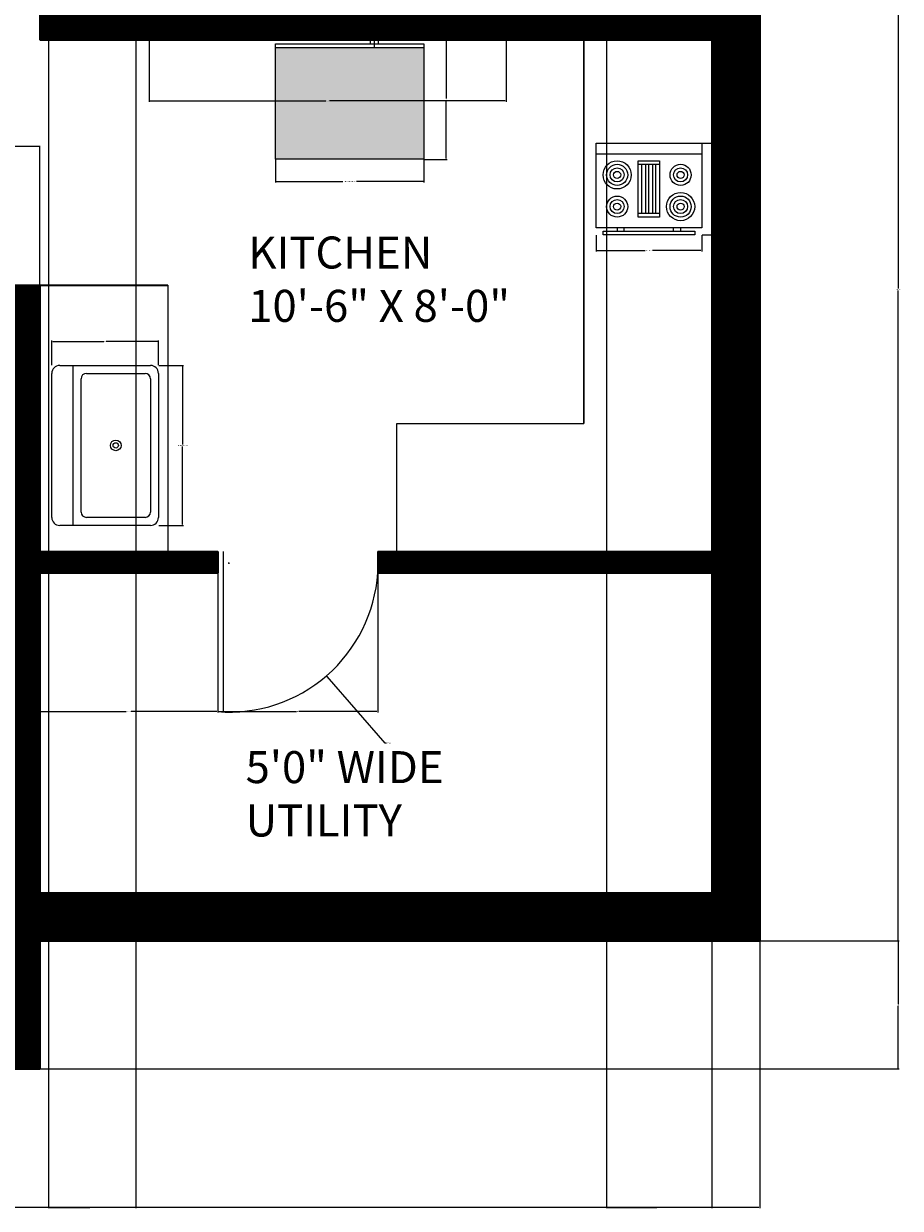
# Model space of a CAD drawing. Units: inches. Extents: x 557 to 1007, y 390 to 953.
# Tile 5 of 10: x 842 to 1007, y 390 to 612. Entities that reach past the tile are written whole.
import ezdxf

# ---------------------------------------------------------------- set-up
doc = ezdxf.new("R2010")
doc.units = ezdxf.units.IN
doc.header["$LTSCALE"] = 5
doc.header["$MEASUREMENT"] = 0
for name, color, linetype, lineweight in [('A-ANNO-DIMS', 2, 'Continuous', 18), ('A-AREA-IDEN', 7, 'Continuous', 18), ('A-DOOR', 3, 'Continuous', 18), ('A-EQPM', 8, 'Continuous', 18), ('A-FLOR-CASE', 8, 'Continuous', 18), ('A-FLOR-FIXT', 9, 'Continuous', 18), ('A-FURN-PATT', 9, 'Continuous', 9), ('A-WALL', 7, 'Continuous', 35)]:
    doc.layers.add(name, color=color, linetype=linetype, lineweight=lineweight)
doc.layers.add('A-GLAZ-PATT', color=141, linetype='Continuous', lineweight=9, true_color=0xadddf7)
doc.layers.add('A-WALL-PATT', color=251, linetype='Continuous', lineweight=9, true_color=0x636466)
doc.styles.get("Standard").update_dxf_attribs({"font": 'arial.ttf'})
doc.dimstyles.get("Standard").update_dxf_attribs({"dimtxt": 0.18, "dimasz": 0.18, "dimexe": 0.18, "dimexo": 0.0625, "dimgap": 0.09, "dimtad": 0, "dimtih": 1, "dimtoh": 1, "dimdec": 4, "dimzin": 0, "dimdsep": 46, "dimtxsty": 'Standard', "dimcen": 0.09, "dimadec": 0, "dimazin": 0, "dimtfac": 1, "dimtdec": 4, "dimtofl": 0, "dimtmove": 0, "dimatfit": 3, "dimfxl": 1, "dimtolj": 1, "dimtzin": 0, "dimarcsym": 0})

# ---------------------------------------------------------------- blocks, each defined once
blk = doc.blocks.new('Refrigerator-2 door - 36 in top')
for p, q in [((0, -26.999999), (36, -26.999999)), ((11, -27.999999), (11, -28.999999)), ((12, -26.999999), (12, -28.999999)), ((13, -28.999999), (13, -27.999999)), ((11, -28.999999), (13, -28.999999))]:
    blk.add_line(p, q)
blk.add_lwpolyline([(0, -27.999999), (0, 0), (36, 0), (36, -27.999999)], close=True)
blk = doc.blocks.new('Sink-single - 30 in top')
blk.add_line((-15, -3.999996), (15, -3.999996))
for points in [[(-13.5, 0), (13.5, 0)], [(-15, -18.499996), (-15, -1.5)], [(15, -1.5), (15, -18.499996)], [(-13.5, -17.499996), (-13.5, -6.499996)], [(-12.5, -5.499996), (12.5, -5.499996)], [(13.5, -6.499996), (13.5, -17.499996)], [(12.5, -18.499996), (-12.5, -18.499996)], [(13.5, -19.999996), (-13.5, -19.999996)]]:
    blk.add_lwpolyline(points)
for radius in [1, 0.5]:
    blk.add_circle((0, -11.999996), radius)
for centre, radius, start, end in [((-13.5, -1.5), 1.5, 90, 180), ((13.5, -1.5), 1.5, 0, 90), ((-12.5, -6.499996), 1, 90, 180), ((12.5, -6.499996), 1, 0, 90), ((-12.5, -17.499996), 1, 180, 270), ((12.5, -17.499996), 1, 270, 0), ((-13.5, -18.499996), 1.5, 180, 270), ((13.5, -18.499996), 1.5, 270, 0)]:
    blk.add_arc(centre, radius, start, end)
blk = doc.blocks.new('Range-Oven - 30 in top')
for p, q in [((0, -3), (30, -3)), ((12, -6), (18, -6)), ((13, -20), (13, -6)), ((14, -6), (14, -20)), ((15, -20), (15, -6)), ((16, -6), (16, -20)), ((17, -20), (17, -6)), ((18, -20), (12, -20)), ((6, -24), (6, -25)), ((8, -25), (8, -24)), ((22, -25), (22, -24)), ((24, -24), (24, -25))]:
    blk.add_line(p, q)
for points in [[(0, -24), (0, 0), (30, 0), (30, -24)], [(12, -21), (12, -5), (18, -5), (18, -21)], [(2, -26), (2, -25), (28, -25), (28, -26)]]:
    blk.add_lwpolyline(points, close=True)
for centre, radius in [((6, -9), 4), ((6, -9), 3), ((24, -9), 3), ((6, -9), 2), ((6, -9), 1), ((24, -9), 2), ((24, -9), 1), ((6, -18), 3), ((6, -18), 2), ((24, -18), 4), ((24, -18), 3), ((24, -18), 2), ((6, -18), 1), ((24, -18), 1)]:
    blk.add_circle(centre, radius)
blk = doc.blocks.new('*D37')
at = {"layer": 'A-ANNO-DIMS', "color": 0, "lineweight": -2, "ltscale": 5, "transparency": 16777216}
for p, q in [((889.59, 586.41), (889.59, 582.12)), ((917.44, 586.41), (917.44, 582.12)), ((889.77, 582.3), (902.26, 582.3)), ((917.26, 582.3), (904.76, 582.3))]:
    blk.add_line(p, q, dxfattribs=at)
at = {"layer": 'A-ANNO-DIMS', "color": 0, "ltscale": 5, "transparency": 16777216}
for points in [[(889.77, 582.33), (889.77, 582.27), (889.59, 582.3)], [(917.26, 582.33), (917.26, 582.27), (917.44, 582.3)]]:
    blk.add_solid(points, dxfattribs=at)
at = {"layer": 'Defpoints', "color": 0, "ltscale": 5, "transparency": 16777216}
for p in [(889.59, 586.47), (917.44, 586.47), (889.59, 582.3)]:
    blk.add_point(p, dxfattribs=at)
at = {"layer": 'A-ANNO-DIMS', "color": 0, "ltscale": 5, "transparency": 16777216, "insert": (903.51, 582.3), "char_height": 0.18, "attachment_point": 5}
blk.add_mtext('\\A1;REFRIGERATOR 28', dxfattribs=at)
blk = doc.blocks.new('*D38')
at = {"layer": 'A-ANNO-DIMS', "color": 0, "lineweight": -2, "ltscale": 5, "transparency": 16777216}
for p, q in [((917.5, 608.9), (921.79, 608.9)), ((921.61, 608.72), (921.61, 597.87)), ((921.61, 586.65), (921.61, 597.51)), ((917.5, 586.47), (921.79, 586.47))]:
    blk.add_line(p, q, dxfattribs=at)
at = {"layer": 'A-ANNO-DIMS', "color": 0, "ltscale": 5, "transparency": 16777216}
for points in [[(921.58, 608.72), (921.64, 608.72), (921.61, 608.9)], [(921.58, 586.65), (921.64, 586.65), (921.61, 586.47)]]:
    blk.add_solid(points, dxfattribs=at)
at = {"layer": 'Defpoints', "color": 0, "ltscale": 5, "transparency": 16777216}
for p in [(917.44, 608.9), (917.44, 586.47), (921.61, 586.47)]:
    blk.add_point(p, dxfattribs=at)
at = {"layer": 'A-ANNO-DIMS', "color": 0, "ltscale": 5, "transparency": 16777216, "insert": (921.61, 597.69), "char_height": 0.18, "attachment_point": 5}
blk.add_mtext('\\A1;22', dxfattribs=at)
blk = doc.blocks.new('*D39')
at = {"layer": 'A-ANNO-DIMS', "color": 0, "lineweight": -2, "ltscale": 5, "transparency": 16777216}
for p, q in [((867.73, 547.83), (872.34, 547.83)), ((872.16, 547.65), (872.16, 533.01)), ((872.16, 518.01), (872.16, 532.64)), ((867.73, 517.83), (872.34, 517.83))]:
    blk.add_line(p, q, dxfattribs=at)
at = {"layer": 'A-ANNO-DIMS', "color": 0, "ltscale": 5, "transparency": 16777216}
for points in [[(872.13, 547.65), (872.19, 547.65), (872.16, 547.83)], [(872.13, 518.01), (872.19, 518.01), (872.16, 517.83)]]:
    blk.add_solid(points, dxfattribs=at)
at = {"layer": 'Defpoints', "color": 0, "ltscale": 5, "transparency": 16777216}
for p in [(867.66, 547.83), (872.16, 547.83), (867.66, 517.83)]:
    blk.add_point(p, dxfattribs=at)
at = {"layer": 'A-ANNO-DIMS', "color": 0, "ltscale": 5, "transparency": 16777216, "insert": (872.16, 532.83), "char_height": 0.18, "attachment_point": 5}
blk.add_mtext('\\A1;KITCHEN SINK 30', dxfattribs=at)
blk = doc.blocks.new('*D40')
at = {"layer": 'A-ANNO-DIMS', "color": 0, "lineweight": -2, "ltscale": 5, "transparency": 16777216}
for p, q in [((847.66, 547.89), (847.66, 552.51)), ((847.84, 552.33), (857.44, 552.33)), ((867.48, 552.33), (857.88, 552.33)), ((867.66, 547.89), (867.66, 552.51))]:
    blk.add_line(p, q, dxfattribs=at)
at = {"layer": 'A-ANNO-DIMS', "color": 0, "ltscale": 5, "transparency": 16777216}
for points in [[(847.84, 552.36), (847.84, 552.3), (847.66, 552.33)], [(867.48, 552.36), (867.48, 552.3), (867.66, 552.33)]]:
    blk.add_solid(points, dxfattribs=at)
at = {"layer": 'Defpoints', "color": 0, "ltscale": 5, "transparency": 16777216}
for p in [(847.66, 552.33), (847.66, 547.83), (867.66, 547.83)]:
    blk.add_point(p, dxfattribs=at)
at = {"layer": 'A-ANNO-DIMS', "color": 0, "ltscale": 5, "transparency": 16777216, "insert": (857.66, 552.33), "char_height": 0.18, "attachment_point": 5}
blk.add_mtext('\\A1;20', dxfattribs=at)
blk = doc.blocks.new('*D41')
at = {"layer": 'A-ANNO-DIMS', "color": 0, "lineweight": -2, "ltscale": 5, "transparency": 16777216}
for p, q in [((949.69, 572.26), (949.69, 569.17)), ((969.5, 572.26), (969.5, 569.17)), ((949.87, 569.35), (958.9, 569.35)), ((969.32, 569.35), (960.29, 569.35))]:
    blk.add_line(p, q, dxfattribs=at)
at = {"layer": 'A-ANNO-DIMS', "color": 0, "ltscale": 5, "transparency": 16777216}
for points in [[(949.87, 569.38), (949.87, 569.32), (949.69, 569.35)], [(969.32, 569.38), (969.32, 569.32), (969.5, 569.35)]]:
    blk.add_solid(points, dxfattribs=at)
at = {"layer": 'Defpoints', "color": 0, "ltscale": 5, "transparency": 16777216}
for p in [(949.69, 572.32), (969.5, 572.32), (969.5, 569.35)]:
    blk.add_point(p, dxfattribs=at)
at = {"layer": 'A-ANNO-DIMS', "color": 0, "ltscale": 5, "transparency": 16777216, "insert": (959.6, 569.35), "char_height": 0.18, "attachment_point": 5}
blk.add_mtext('\\A1;RANGE 20', dxfattribs=at)
blk = doc.blocks.new('*D42')
at = {"layer": 'A-ANNO-DIMS', "color": 0, "lineweight": -2, "ltscale": 5, "transparency": 16777216}
for p, q in [((969.57, 589.5), (972.66, 589.5)), ((972.48, 589.32), (972.48, 581.09)), ((972.48, 572.5), (972.48, 580.73)), ((969.57, 572.32), (972.66, 572.32))]:
    blk.add_line(p, q, dxfattribs=at)
at = {"layer": 'A-ANNO-DIMS', "color": 0, "ltscale": 5, "transparency": 16777216}
for points in [[(972.45, 589.32), (972.51, 589.32), (972.48, 589.5)], [(972.45, 572.5), (972.51, 572.5), (972.48, 572.32)]]:
    blk.add_solid(points, dxfattribs=at)
at = {"layer": 'Defpoints', "color": 0, "ltscale": 5, "transparency": 16777216}
for p in [(969.5, 589.5), (972.48, 589.5), (969.5, 572.32)]:
    blk.add_point(p, dxfattribs=at)
at = {"layer": 'A-ANNO-DIMS', "color": 0, "ltscale": 5, "transparency": 16777216, "insert": (972.48, 580.91), "char_height": 0.18, "attachment_point": 5}
blk.add_mtext('\\A1;17', dxfattribs=at)
blk = doc.blocks.new('*D45')
at = {"layer": 'A-ANNO-DIMS', "color": 0, "lineweight": -2, "ltscale": 5, "transparency": 16777216}
for p, q in [((582.82, 605.84), (582.82, 389.77)), ((980.41, 439.84), (980.41, 389.77)), ((583, 389.95), (781.22, 389.95)), ((980.23, 389.95), (782.01, 389.95))]:
    blk.add_line(p, q, dxfattribs=at)
at = {"layer": 'A-ANNO-DIMS', "color": 0, "ltscale": 5, "transparency": 16777216}
for points in [[(583, 389.98), (583, 389.92), (582.82, 389.95)], [(980.23, 389.98), (980.23, 389.92), (980.41, 389.95)]]:
    blk.add_solid(points, dxfattribs=at)
at = {"layer": 'Defpoints', "color": 0, "ltscale": 5, "transparency": 16777216}
for p in [(582.82, 605.9), (980.41, 439.9), (980.41, 389.95)]:
    blk.add_point(p, dxfattribs=at)
at = {"layer": 'A-ANNO-DIMS', "color": 0, "ltscale": 5, "transparency": 16777216, "insert": (781.61, 389.95), "char_height": 0.18, "attachment_point": 5}
blk.add_mtext('\\A1;397.6', dxfattribs=at)
blk = doc.blocks.new('*D54')
at = {"layer": 'A-ANNO-DIMS', "color": 0, "lineweight": -2, "ltscale": 5, "transparency": 16777216}
for p, q in [((980.47, 439.9), (1006.54, 439.9)), ((1006.36, 439.72), (1006.36, 428.08)), ((1006.36, 416.08), (1006.36, 427.72)), ((845.47, 415.9), (1006.54, 415.9))]:
    blk.add_line(p, q, dxfattribs=at)
at = {"layer": 'A-ANNO-DIMS', "color": 0, "ltscale": 5, "transparency": 16777216}
for points in [[(1006.33, 439.72), (1006.39, 439.72), (1006.36, 439.9)], [(1006.33, 416.08), (1006.39, 416.08), (1006.36, 415.9)]]:
    blk.add_solid(points, dxfattribs=at)
at = {"layer": 'Defpoints', "color": 0, "ltscale": 5, "transparency": 16777216}
for p in [(980.41, 439.9), (1006.36, 439.9), (845.41, 415.9)]:
    blk.add_point(p, dxfattribs=at)
at = {"layer": 'A-ANNO-DIMS', "color": 0, "ltscale": 5, "transparency": 16777216, "insert": (1006.36, 427.9), "char_height": 0.18, "attachment_point": 5}
blk.add_mtext('\\A1;24', dxfattribs=at)
blk = doc.blocks.new('*D55')
at = {"layer": 'A-ANNO-DIMS', "color": 0, "lineweight": -2, "ltscale": 5, "transparency": 16777216}
for p, q in [((980.47, 684.18), (1006.54, 684.18)), ((1006.36, 684), (1006.36, 562.22)), ((1006.36, 440.08), (1006.36, 561.86)), ((980.47, 439.9), (1006.54, 439.9))]:
    blk.add_line(p, q, dxfattribs=at)
at = {"layer": 'A-ANNO-DIMS', "color": 0, "ltscale": 5, "transparency": 16777216}
for points in [[(1006.33, 684), (1006.39, 684), (1006.36, 684.18)], [(1006.33, 440.08), (1006.39, 440.08), (1006.36, 439.9)]]:
    blk.add_solid(points, dxfattribs=at)
at = {"layer": 'Defpoints', "color": 0, "ltscale": 5, "transparency": 16777216}
for p in [(980.41, 684.18), (1006.36, 684.18), (980.41, 439.9)]:
    blk.add_point(p, dxfattribs=at)
at = {"layer": 'A-ANNO-DIMS', "color": 0, "ltscale": 5, "transparency": 16777216, "insert": (1006.36, 562.04), "char_height": 0.18, "attachment_point": 5}
blk.add_mtext('\\A1;244.27', dxfattribs=at)
blk = doc.blocks.new('*D74')
at = {"layer": 'A-ANNO-DIMS', "color": 0, "lineweight": -2, "ltscale": 5, "transparency": 16777216}
for p, q in [((878.77, 508.84), (878.77, 482.77)), ((908.77, 508.84), (908.77, 482.77)), ((878.95, 482.95), (893.55, 482.95)), ((908.59, 482.95), (893.99, 482.95))]:
    blk.add_line(p, q, dxfattribs=at)
at = {"layer": 'A-ANNO-DIMS', "color": 0, "ltscale": 5, "transparency": 16777216}
for points in [[(878.95, 482.98), (878.95, 482.92), (878.77, 482.95)], [(908.59, 482.98), (908.59, 482.92), (908.77, 482.95)]]:
    blk.add_solid(points, dxfattribs=at)
at = {"layer": 'Defpoints', "color": 0, "ltscale": 5, "transparency": 16777216}
for p in [(878.77, 508.9), (908.77, 508.9), (878.77, 482.95)]:
    blk.add_point(p, dxfattribs=at)
at = {"layer": 'A-ANNO-DIMS', "color": 0, "ltscale": 5, "transparency": 16777216, "insert": (893.77, 482.95), "char_height": 0.18, "attachment_point": 5}
blk.add_mtext('\\A1;30', dxfattribs=at)
blk = doc.blocks.new('*D78')
at = {"layer": 'A-ANNO-DIMS', "color": 0, "lineweight": -2, "ltscale": 5, "transparency": 16777216}
for p, q in [((779.41, 562.97), (779.41, 589.03)), ((779.59, 588.85), (812.19, 588.85)), ((845.23, 588.85), (812.62, 588.85)), ((845.41, 562.97), (845.41, 589.03))]:
    blk.add_line(p, q, dxfattribs=at)
at = {"layer": 'A-ANNO-DIMS', "color": 0, "ltscale": 5, "transparency": 16777216}
for points in [[(779.59, 588.88), (779.59, 588.82), (779.41, 588.85)], [(845.23, 588.88), (845.23, 588.82), (845.41, 588.85)]]:
    blk.add_solid(points, dxfattribs=at)
at = {"layer": 'Defpoints', "color": 0, "ltscale": 5, "transparency": 16777216}
for p in [(845.41, 588.85), (779.41, 562.9), (845.41, 562.9)]:
    blk.add_point(p, dxfattribs=at)
at = {"layer": 'A-ANNO-DIMS', "color": 0, "ltscale": 5, "transparency": 16777216, "insert": (812.41, 588.85), "char_height": 0.18, "attachment_point": 5}
blk.add_mtext('\\A1;66', dxfattribs=at)
blk = doc.blocks.new('*D80')
at = {"layer": 'A-ANNO-DIMS', "color": 0, "lineweight": -2, "ltscale": 5, "transparency": 16777216}
for p, q in [((865.93, 623.35), (865.93, 597.28)), ((932.83, 623.35), (932.83, 597.28)), ((866.11, 597.46), (899.06, 597.46)), ((932.65, 597.46), (899.71, 597.46))]:
    blk.add_line(p, q, dxfattribs=at)
at = {"layer": 'A-ANNO-DIMS', "color": 0, "ltscale": 5, "transparency": 16777216}
for points in [[(866.11, 597.49), (866.11, 597.43), (865.93, 597.46)], [(932.65, 597.49), (932.65, 597.43), (932.83, 597.46)]]:
    blk.add_solid(points, dxfattribs=at)
at = {"layer": 'Defpoints', "color": 0, "ltscale": 5, "transparency": 16777216}
for p in [(865.93, 623.41), (932.83, 623.41), (865.93, 597.46)]:
    blk.add_point(p, dxfattribs=at)
at = {"layer": 'A-ANNO-DIMS', "color": 0, "ltscale": 5, "transparency": 16777216, "insert": (899.38, 597.46), "char_height": 0.18, "attachment_point": 5}
blk.add_mtext('\\A1;66.9', dxfattribs=at)
blk = doc.blocks.new('*D84')
at = {"layer": 'A-ANNO-DIMS', "color": 0, "lineweight": -2, "ltscale": 5, "transparency": 16777216}
for p, q in [((847.04, 622.86), (847.04, 389.77)), ((863.45, 622.86), (863.45, 389.77)), ((847.22, 389.95), (854.79, 389.95)), ((863.27, 389.95), (855.7, 389.95))]:
    blk.add_line(p, q, dxfattribs=at)
at = {"layer": 'A-ANNO-DIMS', "color": 0, "ltscale": 5, "transparency": 16777216}
for points in [[(847.22, 389.98), (847.22, 389.92), (847.04, 389.95)], [(863.27, 389.98), (863.27, 389.92), (863.45, 389.95)]]:
    blk.add_solid(points, dxfattribs=at)
at = {"layer": 'Defpoints', "color": 0, "ltscale": 5, "transparency": 16777216}
for p in [(847.04, 622.92), (863.45, 622.92), (863.45, 389.95)]:
    blk.add_point(p, dxfattribs=at)
at = {"layer": 'A-ANNO-DIMS', "color": 0, "ltscale": 5, "transparency": 16777216, "insert": (855.24, 389.95), "char_height": 0.18, "attachment_point": 5}
blk.add_mtext('\\A1;16.408', dxfattribs=at)
blk = doc.blocks.new('*D89')
at = {"layer": 'A-ANNO-DIMS', "color": 0, "lineweight": -2, "ltscale": 5, "transparency": 16777216}
for p, q in [((951.64, 622.86), (951.64, 389.77)), ((971.41, 614.84), (971.41, 389.77)), ((951.82, 389.95), (961.07, 389.95)), ((971.23, 389.95), (961.98, 389.95))]:
    blk.add_line(p, q, dxfattribs=at)
at = {"layer": 'A-ANNO-DIMS', "color": 0, "ltscale": 5, "transparency": 16777216}
for points in [[(951.82, 389.98), (951.82, 389.92), (951.64, 389.95)], [(971.23, 389.98), (971.23, 389.92), (971.41, 389.95)]]:
    blk.add_solid(points, dxfattribs=at)
at = {"layer": 'Defpoints', "color": 0, "ltscale": 5, "transparency": 16777216}
for p in [(951.64, 622.92), (971.41, 614.9), (971.41, 389.95)]:
    blk.add_point(p, dxfattribs=at)
at = {"layer": 'A-ANNO-DIMS', "color": 0, "ltscale": 5, "transparency": 16777216, "insert": (961.52, 389.95), "char_height": 0.18, "attachment_point": 5}
blk.add_mtext('\\A1;19.765', dxfattribs=at)
blk = doc.blocks.new('*D95')
at = {"layer": 'A-ANNO-DIMS', "color": 0, "lineweight": -2, "ltscale": 5, "transparency": 16777216}
for p, q in [((845.41, 508.84), (845.41, 482.77)), ((878.77, 508.84), (878.77, 482.77)), ((845.59, 482.95), (861.62, 482.95)), ((878.59, 482.95), (862.55, 482.95))]:
    blk.add_line(p, q, dxfattribs=at)
at = {"layer": 'A-ANNO-DIMS', "color": 0, "ltscale": 5, "transparency": 16777216}
for points in [[(845.59, 482.98), (845.59, 482.92), (845.41, 482.95)], [(878.59, 482.98), (878.59, 482.92), (878.77, 482.95)]]:
    blk.add_solid(points, dxfattribs=at)
at = {"layer": 'Defpoints', "color": 0, "ltscale": 5, "transparency": 16777216}
for p in [(845.41, 508.9), (878.77, 508.9), (845.41, 482.95)]:
    blk.add_point(p, dxfattribs=at)
at = {"layer": 'A-ANNO-DIMS', "color": 0, "ltscale": 5, "transparency": 16777216, "insert": (862.09, 482.95), "char_height": 0.18, "attachment_point": 5}
blk.add_mtext('\\A1;33.364', dxfattribs=at)
blk = doc.blocks.new('*D96')
at = {"layer": 'A-ANNO-DIMS', "color": 0, "lineweight": -2, "ltscale": 5, "transparency": 16777216}
for p, q in [((947.41, 536.97), (947.41, 953.03)), ((971.41, 512.97), (971.41, 953.03)), ((947.59, 952.85), (959.19, 952.85)), ((971.23, 952.85), (959.63, 952.85))]:
    blk.add_line(p, q, dxfattribs=at)
at = {"layer": 'A-ANNO-DIMS', "color": 0, "ltscale": 5, "transparency": 16777216}
for points in [[(947.59, 952.88), (947.59, 952.82), (947.41, 952.85)], [(971.23, 952.88), (971.23, 952.82), (971.41, 952.85)]]:
    blk.add_solid(points, dxfattribs=at)
at = {"layer": 'Defpoints', "color": 0, "ltscale": 5, "transparency": 16777216}
for p in [(971.41, 952.85), (947.41, 536.9), (971.41, 512.9)]:
    blk.add_point(p, dxfattribs=at)
at = {"layer": 'A-ANNO-DIMS', "color": 0, "ltscale": 5, "transparency": 16777216, "insert": (959.41, 952.85), "char_height": 0.18, "attachment_point": 5}
blk.add_mtext('\\A1;24', dxfattribs=at)
blk = doc.blocks.new('*D110')
at = {"layer": 'A-ANNO-DIMS', "color": 0, "lineweight": -2, "ltscale": 5, "transparency": 16777216}
for p, q in [((880.8, 510.76), (880.98, 510.76)), ((880.89, 510.67), (880.89, 510.85)), ((910.17, 476.98), (899.31, 489.51)), ((910.35, 476.98), (910.17, 476.98))]:
    blk.add_line(p, q, dxfattribs=at)
at = {"layer": 'A-ANNO-DIMS', "color": 0, "ltscale": 5, "transparency": 16777216}
blk.add_solid([(899.33, 489.53), (899.29, 489.49), (899.19, 489.65)], dxfattribs=at)
at = {"layer": 'Defpoints', "color": 0, "ltscale": 5, "transparency": 16777216}
for p in [(880.89, 510.76), (899.19, 489.65)]:
    blk.add_point(p, dxfattribs=at)
at = {"layer": 'A-ANNO-DIMS', "color": 0, "ltscale": 5, "transparency": 16777216, "insert": (910.83, 476.98), "char_height": 0.18, "attachment_point": 5}
blk.add_mtext('\\A1;R27.94', dxfattribs=at)

msp = doc.modelspace()

# ---------------------------------------------------------------- hatches: boundary and pattern name
at = {"layer": 'A-FURN-PATT', "ltscale": 5}
h = msp.add_hatch(dxfattribs=at)
h.set_pattern_fill('GRAVEL', color=256, scale=25)
h.set_pattern_definition([(228.01279, (18, 25), (-200, -225), [3.3634, -332.9772]), (184.96974, (15.75, 22.5), (300, 25), [5.7717, -571.39812]), (132.51045, (10, 22), (250, -275), [4.0697, -402.9008]), (267.27369, (0.25, 15.75), (25, 500), [5.25595, -520.33895]), (292.83365, (0, 10.5), (-125, 300), [5.15387, -510.23433]), (357.27369, (2, 5.75), (-500, 25), [5.25595, -520.33895]), (37.69424, (7.25, 5.5), (-325, -250), [6.95072, -688.1212]), (72.25533, (12.75, 9.75), (175, 550), [6.5622, -649.65804]), (121.42957, (14.75, 16), (-200, 325), [5.27375, -522.10183]), (175.23636, (12, 20.5), (275, -25), [6.0208, -295.01906]), (222.39744, (6, 21), (-300, -275), [7.7862, -770.83438]), (138.81407, (25, 15.5), (-175, 150), [2.65752, -263.0961]), (171.46923, (23, 17.25), (325, -50), [5.05593, -500.5378]), (225, (18, 18), (-3e-15, -25), [3.53552, -31.8198]), (203.1986, (16.25, 21), (125, 50), [1.90395, -188.49038]), (291.8014, (14.5, 20.25), (-25, 75), [2.69257, -131.93655]), (30.96376, (15.5, 17.75), (75, 50), [4.37322, -141.40057]), (161.56505, (19.25, 20), (50, -25), [3.16228, -75.89467]), (16.38954, (0, 20.25), (250, 75), [4.43, -438.57113]), (70.34618, (4.25, 21.5), (-100, -275), [3.71652, -367.9352]), (293.1986, (19.25, 25), (-50, 125), [3.80788, -186.58645]), (343.61046, (20.75, 21.5), (-250, 75), [4.43, -438.57113]), (339.44395, (0, 4.75), (-125, 50), [4.272, -209.3281]), (294.77514, (4, 3.25), (-125, 275), [3.57945, -354.36608]), (66.8014, (19.5, 0), (50, 125), [3.80788, -186.58645]), (17.35402, (21, 3.5), (-325, -100), [4.19078, -414.8856]), (69.44395, (7.25, 0), (-50, -125), [2.136, -211.4641]), (101.30993, (18, 0), (-25, 100), [1.27475, -126.20074]), (165.96376, (17.75, 1.25), (75, -25), [5.15388, -97.92377]), (186.00901, (12.75, 2.5), (250, 25), [4.77625, -472.84808]), (303.69007, (15.5, 15.5), (-25, 50), [3.60555, -86.53323]), (353.15723, (17.5, 12.5), (425, -50), [6.29485, -623.18907]), (60.9454, (23.75, 11.75), (-100, -175), [2.5739, -254.81685]), (90, (25, 14), (-25, 25), [1.5, -23.5]), (120.25644, (12.25, 3.25), (100, -175), [3.4731, -343.838]), (48.01279, (10.5, 6.25), (200, 225), [6.7268, -329.6138]), (0, (15, 11.25), (25, 25), [6.5, -18.5]), (325.30485, (21.5, 11.25), (250, -175), [3.95285, -391.33186]), (254.0546, (24.75, 9), (-25, -100), [3.64005, -178.3627]), (207.64598, (23.75, 5.5), (-475, -250), [5.92662, -586.73685]), (175.42608, (18.5, 2.75), (-325, 25), [6.26997, -620.72684])])
h.paths.add_polyline_path([(615.2525, 688.5, 1), (640.7475, 688.5, 1)])
h.paths.add_polyline_path([(917.0544, 663.8414, 0.33333323), (915.2241, 665.6717), (882.2793, 665.6717, 0.33333323), (880.449, 663.8414), (880.449, 649.1992, 0.33333323), (882.2793, 647.369), (915.2241, 647.369, 0.33333323), (917.0544, 649.1992)])
h.paths.add_polyline_path([(828.0807, 699.7098), (756.0807, 699.7098), (756.0807, 663.7098), (828.0807, 663.7098)])
h.paths.add_polyline_path([(787.5651, 663.7098), (768.5964, 663.7098), (769.8463, 655.7098), (786.3151, 655.7098)])
h.paths.add_polyline_path([(815.5651, 663.7098), (796.5964, 663.7098), (797.8463, 655.7098), (814.3151, 655.7098)])
h.paths.add_polyline_path([(836.0807, 689.9442), (828.0807, 691.1942), (828.0807, 672.2255), (836.0807, 673.4755)])
h.paths.add_polyline_path([(756.0807, 691.1942), (748.0807, 689.9442), (748.0807, 673.4755), (756.0807, 672.2255)])
h.paths.add_polyline_path([(786.3151, 707.7098), (769.8463, 707.7098), (768.5964, 699.7098), (787.5651, 699.7098)])
h.paths.add_polyline_path([(814.3151, 707.7098), (797.8463, 707.7098), (796.5964, 699.7098), (815.5651, 699.7098)])
h.paths.add_polyline_path([(917.4362, 607.3575), (889.5896, 607.3575), (889.5896, 586.4726), (917.4362, 586.4726)])
h.paths.add_polyline_path([(721.4053, 881.8539), (671.0053, 881.8539), (671.0053, 866.6539), (658.2053, 866.6539), (658.2053, 821.8539), (721.4053, 821.8539)])
h.paths.add_polyline_path([(925.4053, 875.1046), (875.0053, 875.1046), (875.0053, 859.9046), (862.2053, 859.9046), (862.2053, 815.1046), (925.4053, 815.1046)])
h.paths.add_polyline_path([(721.4053, 558.9046), (671.0053, 558.9046), (671.0053, 543.7046), (658.2053, 543.7046), (658.2053, 498.9046), (721.4053, 498.9046)])
at = {"layer": 'A-FURN-PATT'}
h = msp.add_hatch(dxfattribs=at)
h.set_pattern_fill('CROSS', color=256, scale=25)
h.paths.add_polyline_path([(925.4053, 875.1046), (875.0053, 875.1046), (875.0053, 859.9046), (862.2053, 859.9046), (862.2053, 815.1046), (925.4053, 815.1046)])
h.paths.add_polyline_path([(721.4053, 881.8539), (671.0053, 881.8539), (671.0053, 866.6539), (658.2053, 866.6539), (658.2053, 821.8539), (721.4053, 821.8539)])
h.paths.add_polyline_path([(671.0053, 881.8539), (655.8053, 866.6539), (671.0053, 866.6539)], flags=17)
h.paths.add_polyline_path([(671.0053, 881.8539), (641.4053, 881.8539), (641.4053, 821.8539), (655.8053, 821.8539), (655.8053, 829.8539), (642.6053, 829.8539), (642.6053, 850.6539), (655.8053, 850.6539), (655.8053, 853.0539), (642.6053, 853.0539), (642.6053, 873.8539), (657.8053, 873.8539), (657.8053, 868.6539)])
h.paths.add_polyline_path([(875.0053, 875.1046), (859.8053, 859.9046), (875.0053, 859.9046)], flags=17)
h.paths.add_polyline_path([(875.0053, 875.1046), (845.4053, 875.1046), (845.4053, 815.1046), (859.8053, 815.1046), (859.8053, 823.1046), (846.6053, 823.1046), (846.6053, 843.9046), (859.8053, 843.9046), (859.8053, 846.3046), (846.6053, 846.3046), (846.6053, 867.1046), (861.8053, 867.1046), (861.8053, 861.9046)])
h.paths.add_polyline_path([(721.4053, 558.9046), (671.0053, 558.9046), (671.0053, 543.7046), (658.2053, 543.7046), (658.2053, 498.9046), (721.4053, 498.9046)])
h.paths.add_polyline_path([(671.0053, 558.9046), (641.4053, 558.9046), (641.4053, 498.9046), (655.8053, 498.9046), (655.8053, 506.9046), (642.6053, 506.9046), (642.6053, 527.7046), (655.8053, 527.7046), (655.8053, 530.1046), (642.6053, 530.1046), (642.6053, 550.9046), (657.8053, 550.9046), (657.8053, 545.7046)])
h.paths.add_polyline_path([(671.0053, 558.9046), (657.8053, 545.7046), (655.8053, 543.7046), (671.0053, 543.7046)], flags=17)
h.paths.add_polyline_path([(873.1461, 661.8773, 0.41421356), (868.1461, 666.8773, -0.12244426), (867.1516, 666.8773), (855.014, 666.8773), (855.014, 647.2429), (867.4581, 647.2429, -0.08537395), (868.1461, 647.2429, 0.41421356), (873.1461, 652.2429)])
h.paths.add_polyline_path([(917.0544, 663.8414, 0.33333323), (915.2241, 665.6717), (882.2793, 665.6717, 0.33333323), (880.449, 663.8414), (880.449, 649.1992, 0.33333323), (882.2793, 647.369), (915.2241, 647.369, 0.33333323), (917.0544, 649.1992)])
h.paths.add_polyline_path([(944.9465, 667.5202), (932.6561, 667.5202, -0.10407786), (931.8144, 667.5202, 0.41421356), (926.8144, 662.5202), (926.8144, 652.8858, 0.41421356), (931.8144, 647.8858, -0.05611627), (932.2647, 647.8858), (944.9465, 647.8858)])
h.paths.add_polyline_path([(928.8341, 635.542, 0.41421356), (923.8341, 640.542), (914.1997, 640.542, 0.41421356), (909.1997, 635.542), (909.1997, 622.4099), (923.8341, 622.4099, 0.41421356), (928.8341, 627.4099)])
h.paths.add_polyline_path([(909.1997, 635.542, 0.41421356), (904.1997, 640.542), (894.5653, 640.542, 0.41421356), (889.5653, 635.542), (889.5653, 622.4099), (909.1997, 622.4099)])
h.paths.add_polyline_path([(889.5653, 635.542, 0.41421356), (884.5653, 640.542), (874.9308, 640.542, 0.41421356), (869.9308, 635.542), (869.9308, 627.4099, 0.41421356), (874.9308, 622.4099), (889.5653, 622.4099)])
at = {"layer": 'A-GLAZ-PATT'}
h = msp.add_hatch(dxfattribs=at)
h.set_pattern_fill('ANSI31', color=256)
h.paths.add_polyline_path([(635.9053, 814.7688), (636.9053, 814.7688), (636.9053, 838.7688), (632.4053, 838.7688), (632.4053, 790.7688), (635.9053, 790.7688)])
h.paths.add_polyline_path([(641.4053, 838.7688), (637.9053, 838.7688), (637.9053, 814.7688), (636.9053, 814.7688), (636.9053, 790.7688), (641.4053, 790.7688)])
h.paths.add_polyline_path([(603.4053, 728.9046, -0.41421356), (623.4053, 748.9046), (632.4053, 748.9046), (632.4053, 752.9046), (623.4053, 752.9046, 0.41421356), (599.4053, 728.9046), (599.4053, 614.9046), (603.4053, 614.9046)])
h.paths.add_polyline_path([(632.4053, 743.9046), (632.4053, 747.9046), (623.4053, 747.9046, 0.41421356), (604.4053, 728.9046), (604.4053, 614.9046), (608.4053, 614.9046), (608.4053, 719.9046, -0.41421356)])
h.paths.add_polyline_path([(683.4053, 722.9046), (678.9053, 722.9046), (678.9053, 698.9046), (679.9053, 698.9046), (679.9053, 662.9046), (678.9053, 662.9046), (678.9053, 638.9046), (683.4053, 638.9046)])
h.paths.add_polyline_path([(678.9053, 698.9046), (677.9053, 698.9046), (677.9053, 722.9046), (674.4053, 722.9046), (674.4053, 638.9046), (677.9053, 638.9046), (677.9053, 662.9046), (678.9053, 662.9046)])
h.paths.add_polyline_path([(635.9053, 593.9046), (632.4053, 593.9046), (632.4053, 557.9046), (635.9053, 557.9046)])
h.paths.add_polyline_path([(641.4053, 593.9046), (637.9053, 593.9046), (637.9053, 557.9046), (641.4053, 557.9046)])
h.paths.add_polyline_path([(764.9579, 448.9046), (716.9579, 448.9046), (716.9579, 445.4046), (740.9579, 445.4046), (740.9579, 444.4046), (764.9579, 444.4046)])
h.paths.add_polyline_path([(764.9579, 443.4046), (740.9579, 443.4046), (740.9579, 444.4046), (716.9579, 444.4046), (716.9579, 439.9046), (764.9579, 439.9046)])
h.paths.add_polyline_path([(938.4053, 905.9046), (878.4053, 905.9046), (878.4053, 902.4046), (908.4053, 902.4046), (908.4053, 901.4046), (938.4053, 901.4046)])
h.paths.add_polyline_path([(938.4053, 900.4046), (908.4053, 900.4046), (908.4053, 901.4046), (878.4053, 901.4046), (878.4053, 896.9046), (938.4053, 896.9046)])
h.paths.add_polyline_path([(724.9087, 905.9046), (676.9087, 905.9046), (676.9087, 902.4046), (701.4053, 902.4046), (701.4053, 901.4046), (724.9087, 901.4046)])
h.paths.add_polyline_path([(724.9087, 900.4046), (701.4053, 900.4046), (701.4053, 901.4046), (676.9087, 901.4046), (676.9087, 896.9046), (724.9087, 896.9046)])
h.paths.add_polyline_path([(832.0625, 905.9046), (808.0625, 905.9046), (808.0625, 902.4046), (832.0625, 902.4046)])
h.paths.add_polyline_path([(832.0625, 900.4046), (808.0625, 900.4046), (808.0625, 896.9046), (832.0625, 896.9046)])
at = {"layer": 'A-WALL-PATT'}
h = msp.add_hatch(dxfattribs=at)
h.set_pattern_fill('ANSI31', color=256)
h.paths.add_polyline_path([(808.0625, 905.9046), (767.4053, 905.9046), (767.4053, 920.9046), (839.4053, 920.9046), (839.4053, 905.9046), (832.0625, 905.9046), (832.0625, 896.9046), (839.4053, 896.9046), (839.4053, 800.9046), (837.4053, 800.9046), (837.4053, 794.9046), (839.4053, 794.9046), (839.4053, 790.9046), (845.4053, 790.9046), (845.4053, 896.9046), (878.4053, 896.9046), (878.4053, 905.9046), (845.4053, 905.9046), (845.4053, 926.9046), (761.4053, 926.9046), (761.4053, 914.9046), (761.4053, 905.9046), (724.9087, 905.9046), (724.9087, 896.9046), (761.4053, 896.9046), (761.4053, 752.9046), (759.4053, 752.9046), (759.4053, 746.9046), (767.4053, 746.9046), (767.4053, 794.9046), (807.4053, 794.9046), (807.4053, 800.9046), (767.4053, 800.9046), (767.4053, 896.9046), (808.0625, 896.9046)])
h.paths.add_polyline_path([(676.9087, 905.9046), (632.4053, 905.9046), (632.4053, 838.7688), (641.4053, 838.7688), (641.4053, 881.8539), (641.4053, 896.9046), (676.9087, 896.9046)])
h.paths.add_polyline_path([(980.4053, 905.9046), (938.4053, 905.9046), (938.4053, 896.9046), (971.4053, 896.9046), (971.4053, 752.9046), (845.4053, 752.9046), (845.4053, 754.9046), (839.4053, 754.9046), (839.4053, 746.9046), (971.4053, 746.9046), (971.4053, 720.1788), (980.4053, 720.1788)])
h.paths.add_polyline_path([(723.4053, 752.9046), (641.4053, 752.9046), (641.4053, 790.7688), (632.4053, 790.7688), (632.4053, 743.9046), (674.4053, 743.9046), (674.4053, 722.9046), (683.4053, 722.9046), (683.4053, 746.9046), (723.4053, 746.9046)])
h.paths.add_polyline_path([(980.4053, 684.1788), (971.4053, 684.1788), (971.4053, 614.9046), (845.4053, 614.9046), (845.4053, 608.9046), (971.4053, 608.9046), (971.4053, 512.9046), (908.7697, 512.9046), (908.7697, 508.9046), (971.4053, 508.9046), (971.4053, 448.9046), (845.4053, 448.9046), (845.4053, 508.9046), (878.7697, 508.9046), (878.7697, 512.9046), (845.4053, 512.9046), (845.4053, 562.9046), (779.4053, 562.9046), (779.4053, 614.9046), (761.4053, 614.9046), (761.4053, 608.9046), (773.4053, 608.9046), (773.4053, 512.636), (779.4053, 512.636), (779.4053, 556.9046), (839.4053, 556.9046), (839.4053, 448.9046), (830.432, 448.9046), (830.432, 439.9046), (839.4053, 439.9046), (839.4053, 433.0506), (839.4053, 421.9046), (779.4053, 421.9046), (779.4053, 439.9046), (796.9656, 439.9046), (806.432, 439.9046), (806.432, 448.9046), (779.4053, 448.9046), (779.4053, 482.636), (773.4053, 482.636), (773.4053, 448.9046), (764.9579, 448.9046), (764.9579, 439.9046), (773.4053, 439.9046), (773.4053, 415.9046), (845.4053, 415.9046), (845.4053, 439.9046), (980.4053, 439.9046)])
h.paths.add_polyline_path([(716.9579, 448.9046), (641.4053, 448.9046), (641.4053, 557.9046), (632.4053, 557.9046), (632.4053, 439.9046), (716.9579, 439.9046)])
h.paths.add_polyline_path([(725.4053, 614.9046), (683.4053, 614.9046), (683.4053, 638.9046), (674.4053, 638.9046), (674.4053, 614.9046), (608.4053, 614.9046), (582.8236, 614.9046), (582.8236, 605.9046), (599.4053, 605.9046), (632.4053, 605.9046), (641.4053, 605.9046), (641.4053, 608.9046), (725.4053, 608.9046)])
h.paths.add_polyline_path([(641.4053, 605.9046), (632.4053, 605.9046), (632.4053, 593.9046), (641.4053, 593.9046)])

# ---------------------------------------------------------------- linework, layer by layer
at = {"layer": 'A-DOOR'}
for p, q in [((878.7697, 512.9046), (878.7697, 482.9046)), ((879.7697, 512.9046), (879.7697, 482.9046))]:
    msp.add_line(p, q, dxfattribs=at)
msp.add_arc((880.8934, 510.7619), 27.9381, 265.640561, 356.188206, dxfattribs=at)
at = {"layer": 'A-FLOR-CASE'}
for p, q in [((947.4053, 608.9046), (947.4053, 536.9046)), ((869.4053, 562.9046), (869.4053, 512.9046)), ((912.3462, 536.9046), (947.4053, 536.9046)), ((912.3462, 512.9046), (912.3462, 536.9046))]:
    msp.add_line(p, q, dxfattribs=at)
at = {"layer": 'A-WALL'}
for p, q in [((980.4053, 684.1788), (980.4053, 439.9046)), ((845.4053, 614.9046), (845.4053, 608.9046)), ((845.4053, 608.9046), (971.4053, 608.9046)), ((971.4053, 608.9046), (971.4053, 512.9046)), ((779.4053, 562.9046), (869.4053, 562.9046)), ((845.4053, 562.9046), (845.4053, 512.9046)), ((845.4053, 512.9046), (878.7697, 512.9046)), ((878.7697, 512.9046), (878.7697, 508.9046)), ((908.7697, 512.9046), (908.7697, 508.9046)), ((908.7697, 512.9046), (971.4053, 512.9046)), ((845.4053, 508.9046), (878.7697, 508.9046)), ((845.4053, 508.9046), (845.4053, 448.9046)), ((908.7697, 508.9046), (971.4053, 508.9046)), ((971.4053, 508.9046), (971.4053, 448.9046)), ((845.4053, 448.9046), (971.4053, 448.9046)), ((845.4053, 439.9046), (845.4053, 415.9046)), ((845.4053, 439.9046), (980.4053, 439.9046)), ((773.4053, 415.9046), (845.4053, 415.9046))]:
    msp.add_line(p, q, dxfattribs=at)

# ---------------------------------------------------------------- block references
at = {"layer": 'A-EQPM', "xscale": 0.7735177963891468, "yscale": 0.7735177963891468, "zscale": 0.7735177963891468, "rotation": 180}
msp.add_blockref('Refrigerator-2 door - 36 in top', (917.4362, 586.4726), dxfattribs=at)
at = {"layer": 'A-EQPM', "xscale": 0.6605650799146243, "yscale": 0.6605650799146243, "zscale": 0.6605650799146243}
msp.add_blockref('Range-Oven - 30 in top', (949.687, 589.4993), dxfattribs=at)
at = {"layer": 'A-FLOR-FIXT', "rotation": 90}
msp.add_blockref('Sink-single - 30 in top', (847.6635, 532.8257), dxfattribs=at)

# ---------------------------------------------------------------- texts
at = {"layer": 'A-AREA-IDEN', "char_height": 6, "attachment_point": 1}
for s, insert in [('KITCHEN\\P10\'-6" X 8\'-0"', (884.5, 572)), ('5\'0" WIDE \\PUTILITY', (884, 475.5))]:
    msp.add_mtext_dynamic_manual_height_columns(s, width=125, gutter_width=1, heights=[0], dxfattribs=dict(at, insert=insert))

# ---------------------------------------------------------------- dimensions: what is measured, and where the dimension line sits
at = {"layer": 'A-ANNO-DIMS', "ltscale": 5}
for base, p1, p2, override, picture, middle in [((971.4053, 952.8546), (947.4053, 536.9046), (971.4053, 512.9046), {"dimdec": 0, "dimlfac": 1, "dimrnd": 0, "dimzin": 0, "dimdsep": 46, "dimlunit": 2}, '*D96', (959.4053, 952.8546)), ((863.4458, 389.9546), (847.0376, 622.9231), (863.4458, 622.9231), {"dimdec": 3, "dimlfac": 1, "dimrnd": 0, "dimzin": 0, "dimdsep": 46, "dimlunit": 2}, '*D84', (855.2417, 389.9546)), ((971.4053, 389.9546), (951.6399, 622.9231), (971.4053, 614.9046), {"dimdec": 3, "dimlfac": 1, "dimrnd": 0, "dimzin": 0, "dimdsep": 46, "dimlunit": 2}, '*D89', (961.5226, 389.9546)), ((980.4053, 389.9546), (582.8236, 605.9046), (980.4053, 439.9046), {"dimdec": 1, "dimlfac": 1, "dimrnd": 0, "dimzin": 0, "dimdsep": 46, "dimlunit": 2}, '*D45', (781.6144, 389.9546))]:
    dim = msp.add_linear_dim(base=base, p1=p1, p2=p2, dimstyle='Standard', override=override, dxfattribs=at)
    dim.commit()
    dim.dimension.update_dxf_attribs({"geometry": picture, "text_midpoint": middle})
for base, p1, p2, angle, override, picture, middle in [((1006.3553, 684.1788), (980.4053, 439.9046), (980.4053, 684.1788), 90, {"dimdec": 2, "dimlfac": 1, "dimrnd": 0, "dimzin": 0, "dimdsep": 46, "dimlunit": 2}, '*D55', (1006.3553, 562.0417)), ((865.9308, 597.4599), (932.8341, 623.4099), (865.9308, 623.4099), 180, {"dimdec": 1, "dimlfac": 1, "dimrnd": 0, "dimzin": 0, "dimdsep": 46, "dimlunit": 2}, '*D80', (899.3825, 597.4599)), ((921.6132, 586.4726), (917.4362, 608.9046), (917.4362, 586.4726), 270, {"dimdec": 0, "dimlfac": 1, "dimrnd": 0, "dimzin": 0, "dimdsep": 46, "dimlunit": 2}, '*D38', (921.6132, 597.6886)), ((845.4053, 588.8546), (779.4053, 562.9046), (845.4053, 562.9046), 0, {"dimdec": 0, "dimlfac": 1, "dimrnd": 0, "dimzin": 0, "dimdsep": 46, "dimlunit": 2}, '*D78', (812.4053, 588.8546)), ((972.4765, 589.4993), (969.5039, 572.3246), (969.5039, 589.4993), 90, {"dimdec": 0, "dimlfac": 1, "dimrnd": 0, "dimzin": 0, "dimdsep": 46, "dimlunit": 2}, '*D42', (972.4765, 580.912)), ((847.6635, 552.3257), (867.6635, 547.8257), (847.6635, 547.8257), 180, {"dimdec": 0, "dimlfac": 1, "dimrnd": 0, "dimzin": 0, "dimdsep": 46, "dimlunit": 2}, '*D40', (857.6635, 552.3257)), ((845.4053, 482.9546), (878.7697, 508.9046), (845.4053, 508.9046), 180, {"dimdec": 3, "dimlfac": 1, "dimrnd": 0, "dimzin": 0, "dimdsep": 46, "dimlunit": 2}, '*D95', (862.0875, 482.9546)), ((878.7697, 482.9546), (908.7697, 508.9046), (878.7697, 508.9046), 180, {"dimdec": 0, "dimlfac": 1, "dimrnd": 0, "dimzin": 0, "dimdsep": 46, "dimlunit": 2}, '*D74', (893.7697, 482.9546)), ((1006.3553, 439.9046), (845.4053, 415.9046), (980.4053, 439.9046), 90, {"dimdec": 0, "dimlfac": 1, "dimrnd": 0, "dimzin": 0, "dimdsep": 46, "dimlunit": 2}, '*D54', (1006.3553, 427.9046))]:
    dim = msp.add_linear_dim(base=base, p1=p1, p2=p2, angle=angle, dimstyle='Standard', override=override, dxfattribs=at)
    dim.commit()
    dim.dimension.update_dxf_attribs({"geometry": picture, "text_midpoint": middle})
for base, p1, p2, angle, text, picture, middle in [((889.5896, 582.2956), (917.4362, 586.4726), (889.5896, 586.4726), 180, 'REFRIGERATOR <>', '*D37', (903.5129, 582.2956)), ((872.1635, 547.8257), (867.6635, 517.8257), (867.6635, 547.8257), 90, 'KITCHEN SINK <>', '*D39', (872.1635, 532.8257))]:
    dim = msp.add_linear_dim(base=base, p1=p1, p2=p2, angle=angle, text=text, dimstyle='Standard', override={"dimdec": 0, "dimlfac": 1, "dimrnd": 0, "dimzin": 0, "dimdsep": 46, "dimlunit": 2}, dxfattribs=at)
    dim.commit()
    dim.dimension.update_dxf_attribs({"geometry": picture, "text_midpoint": middle})
dim = msp.add_linear_dim(base=(969.5039, 569.3521), p1=(949.687, 572.3246), p2=(969.5039, 572.3246), text='RANGE <>', dimstyle='Standard', override={"dimdec": 0, "dimlfac": 1, "dimrnd": 0, "dimzin": 0, "dimdsep": 46, "dimlunit": 2}, dxfattribs=at)
dim.commit()
dim.dimension.update_dxf_attribs({"geometry": '*D41', "text_midpoint": (959.5955, 569.3521)})
dim = msp.add_radius_dim(center=(880.8934, 510.7619), mpoint=(899.1908, 489.6492), dimstyle='Standard', override={"dimdec": 2, "dimlfac": 1, "dimrnd": 0, "dimzin": 0, "dimdsep": 46, "dimlunit": 2}, dxfattribs=at)
dim.commit()
dim.dimension.update_dxf_attribs({"geometry": '*D110', "text_midpoint": (910.8287, 476.9817), "dimtype": 164})

doc.saveas('drawing.dxf')
